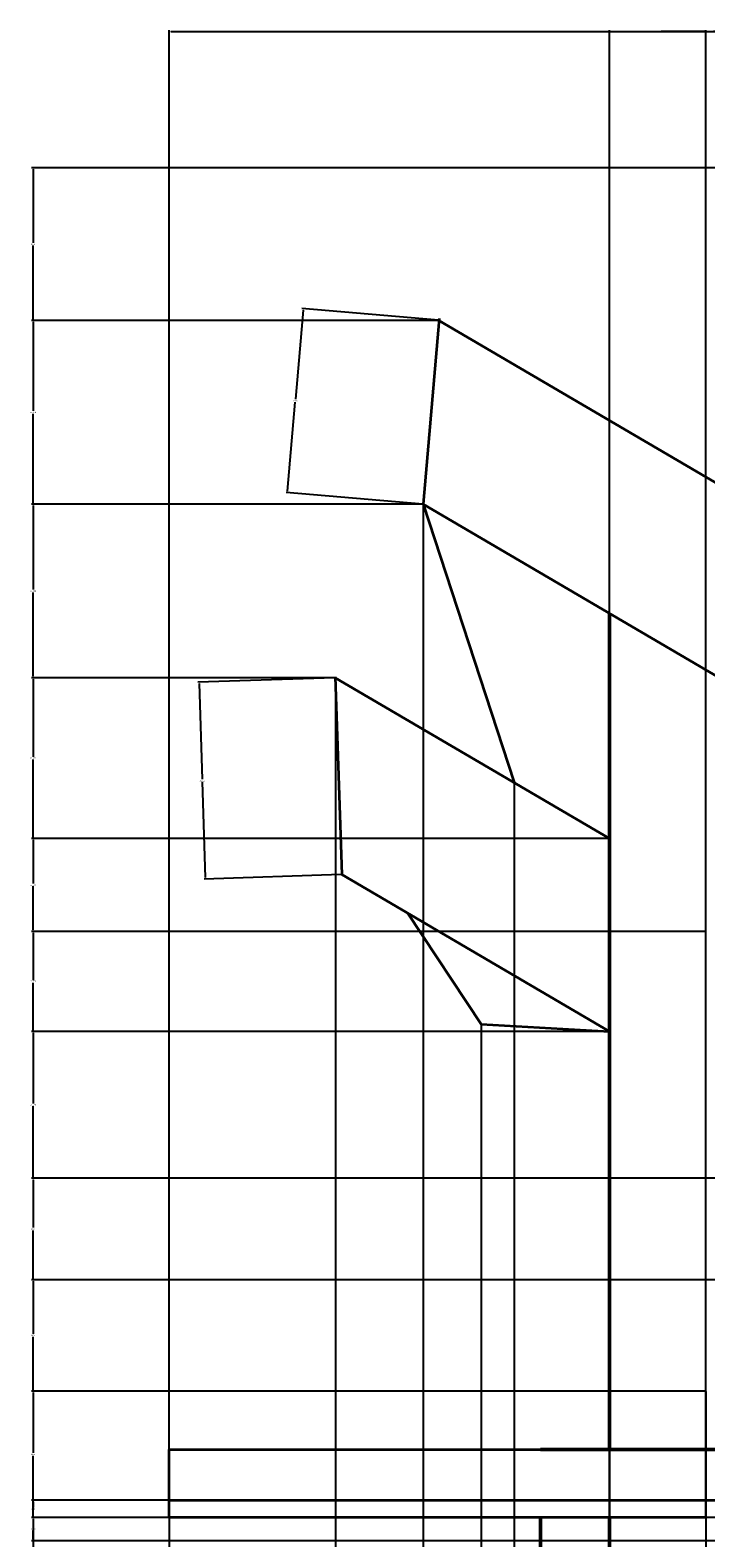
# Model space of a CAD drawing. Units: inches. Extents: x 27 to 409, y -26 to 294.
# Tile 3 of 7: x 27 to 116, y 97 to 294. Entities that reach past the tile are written whole.
import ezdxf

# ---------------------------------------------------------------- set-up
doc = ezdxf.new("R2010")
doc.units = ezdxf.units.IN
doc.header["$MEASUREMENT"] = 0
for name, color, linetype, lineweight in [('A-ANNO-DIMS', 2, 'Continuous', 18), ('A-ROOF', 1, 'Continuous', 35), ('A-WALL', 7, 'Continuous', 50)]:
    doc.layers.add(name, color=color, linetype=linetype, lineweight=lineweight)
doc.styles.get("Standard").update_dxf_attribs({"font": 'arial.ttf'})
doc.dimstyles.get("Standard").update_dxf_attribs({"dimtxt": 0.18, "dimasz": 0.18, "dimexe": 0.18, "dimexo": 0.0625, "dimgap": 0.09, "dimtad": 0, "dimtih": 1, "dimtoh": 1, "dimdec": 4, "dimzin": 0, "dimdsep": 46, "dimtxsty": 'Standard', "dimcen": 0.09, "dimadec": 0, "dimazin": 0, "dimtfac": 1, "dimtdec": 4, "dimtofl": 0, "dimtmove": 0, "dimatfit": 3, "dimfxl": 1, "dimtolj": 1, "dimtzin": 0, "dimarcsym": 0})

# ---------------------------------------------------------------- blocks, each defined once
blk = doc.blocks.new('*D7')
at = {"layer": 'A-ANNO-DIMS', "color": 0, "lineweight": -2, "transparency": 16777216}
for p, q in [((45.58, 108.44), (45.58, 293.63)), ((45.76, 293.45), (217.77, 293.45)), ((390.53, 293.45), (218.52, 293.45)), ((390.71, 136.32), (390.71, 293.63))]:
    blk.add_line(p, q, dxfattribs=at)
at = {"layer": 'A-ANNO-DIMS', "color": 0, "transparency": 16777216}
for points in [[(45.76, 293.48), (45.76, 293.42), (45.58, 293.45)], [(390.53, 293.48), (390.53, 293.42), (390.71, 293.45)]]:
    blk.add_solid(points, dxfattribs=at)
at = {"layer": 'Defpoints', "color": 0, "transparency": 16777216}
for p in [(390.71, 293.45), (390.71, 136.26), (45.58, 108.38)]:
    blk.add_point(p, dxfattribs=at)
at = {"layer": 'A-ANNO-DIMS', "color": 0, "transparency": 16777216, "insert": (218.14, 293.45), "char_height": 0.18, "attachment_point": 5}
blk.add_mtext('\\A1;345.1', dxfattribs=at)
blk = doc.blocks.new('*D8')
at = {"layer": 'A-ANNO-DIMS', "color": 0, "lineweight": -2, "transparency": 16777216}
for p, q in [((67.27, 209.05), (67.27, -26.5)), ((45.58, 99.43), (45.58, -26.5)), ((45.76, -26.32), (56.03, -26.32)), ((67.09, -26.32), (56.82, -26.32))]:
    blk.add_line(p, q, dxfattribs=at)
at = {"layer": 'A-ANNO-DIMS', "color": 0, "transparency": 16777216}
for points in [[(45.76, -26.29), (45.76, -26.35), (45.58, -26.32)], [(67.09, -26.29), (67.09, -26.35), (67.27, -26.32)]]:
    blk.add_solid(points, dxfattribs=at)
at = {"layer": 'Defpoints', "color": 0, "transparency": 16777216}
for p in [(67.27, 209.11), (45.58, 99.5), (67.27, -26.32)]:
    blk.add_point(p, dxfattribs=at)
at = {"layer": 'A-ANNO-DIMS', "color": 0, "transparency": 16777216, "insert": (56.42, -26.32), "char_height": 0.18, "attachment_point": 5}
blk.add_mtext('\\A1;21.69', dxfattribs=at)
blk = doc.blocks.new('*D9')
at = {"layer": 'A-ANNO-DIMS', "color": 0, "lineweight": -2, "transparency": 16777216}
for p, q in [((78.75, 231.7), (78.75, -26.5)), ((67.27, 209.05), (67.27, -26.5)), ((67.45, -26.32), (72.55, -26.32)), ((78.57, -26.32), (73.46, -26.32))]:
    blk.add_line(p, q, dxfattribs=at)
at = {"layer": 'A-ANNO-DIMS', "color": 0, "transparency": 16777216}
for points in [[(67.45, -26.29), (67.45, -26.35), (67.27, -26.32)], [(78.57, -26.29), (78.57, -26.35), (78.75, -26.32)]]:
    blk.add_solid(points, dxfattribs=at)
at = {"layer": 'Defpoints', "color": 0, "transparency": 16777216}
for p in [(78.75, 231.76), (67.27, 209.11), (78.75, -26.32)]:
    blk.add_point(p, dxfattribs=at)
at = {"layer": 'A-ANNO-DIMS', "color": 0, "transparency": 16777216, "insert": (73.01, -26.32), "char_height": 0.18, "attachment_point": 5}
blk.add_mtext('\\A1;11.482', dxfattribs=at)
blk = doc.blocks.new('*D10')
at = {"layer": 'A-ANNO-DIMS', "color": 0, "lineweight": -2, "transparency": 16777216}
for p, q in [((78.75, 231.7), (78.75, -26.5)), ((81.81, -8.58), (81.81, -26.5)), ((78.93, -26.32), (79.89, -26.32)), ((81.63, -26.32), (80.68, -26.32))]:
    blk.add_line(p, q, dxfattribs=at)
at = {"layer": 'A-ANNO-DIMS', "color": 0, "transparency": 16777216}
for points in [[(78.93, -26.29), (78.93, -26.35), (78.75, -26.32)], [(81.63, -26.29), (81.63, -26.35), (81.81, -26.32)]]:
    blk.add_solid(points, dxfattribs=at)
at = {"layer": 'Defpoints', "color": 0, "transparency": 16777216}
for p in [(78.75, 231.76), (81.81, -8.52), (81.81, -26.32)]:
    blk.add_point(p, dxfattribs=at)
at = {"layer": 'A-ANNO-DIMS', "color": 0, "transparency": 16777216, "insert": (80.28, -26.32), "char_height": 0.18, "attachment_point": 5}
blk.add_mtext('\\A1;3.064', dxfattribs=at)
blk = doc.blocks.new('*D11')
at = {"layer": 'A-ANNO-DIMS', "color": 0, "lineweight": -2, "transparency": 16777216}
for p, q in [((86.32, 163.84), (86.32, -26.5)), ((81.81, -8.58), (81.81, -26.5)), ((81.99, -26.32), (83.67, -26.32)), ((86.14, -26.32), (84.46, -26.32))]:
    blk.add_line(p, q, dxfattribs=at)
at = {"layer": 'A-ANNO-DIMS', "color": 0, "transparency": 16777216}
for points in [[(81.99, -26.29), (81.99, -26.35), (81.81, -26.32)], [(86.14, -26.29), (86.14, -26.35), (86.32, -26.32)]]:
    blk.add_solid(points, dxfattribs=at)
at = {"layer": 'Defpoints', "color": 0, "transparency": 16777216}
for p in [(86.32, 163.9), (81.81, -8.52), (86.32, -26.32)]:
    blk.add_point(p, dxfattribs=at)
at = {"layer": 'A-ANNO-DIMS', "color": 0, "transparency": 16777216, "insert": (84.07, -26.32), "char_height": 0.18, "attachment_point": 5}
blk.add_mtext('\\A1;4.503', dxfattribs=at)
blk = doc.blocks.new('*D12')
at = {"layer": 'A-ANNO-DIMS', "color": 0, "lineweight": -2, "transparency": 16777216}
for p, q in [((90.63, 195.36), (90.63, -26.5)), ((86.32, 163.84), (86.32, -26.5)), ((86.5, -26.32), (88.09, -26.32)), ((90.45, -26.32), (88.85, -26.32))]:
    blk.add_line(p, q, dxfattribs=at)
at = {"layer": 'A-ANNO-DIMS', "color": 0, "transparency": 16777216}
for points in [[(86.5, -26.29), (86.5, -26.35), (86.32, -26.32)], [(90.45, -26.29), (90.45, -26.35), (90.63, -26.32)]]:
    blk.add_solid(points, dxfattribs=at)
at = {"layer": 'Defpoints', "color": 0, "transparency": 16777216}
for p in [(90.63, 195.42), (86.32, 163.9), (90.63, -26.32)]:
    blk.add_point(p, dxfattribs=at)
at = {"layer": 'A-ANNO-DIMS', "color": 0, "transparency": 16777216, "insert": (88.47, -26.32), "char_height": 0.18, "attachment_point": 5}
blk.add_mtext('\\A1;4.311', dxfattribs=at)
blk = doc.blocks.new('*D13')
at = {"layer": 'A-ANNO-DIMS', "color": 0, "lineweight": -2, "transparency": 16777216}
for p, q in [((90.63, 195.36), (90.63, -26.5)), ((103.08, 162.87), (103.08, -26.5)), ((90.81, -26.32), (96.4, -26.32)), ((102.9, -26.32), (97.31, -26.32))]:
    blk.add_line(p, q, dxfattribs=at)
at = {"layer": 'A-ANNO-DIMS', "color": 0, "transparency": 16777216}
for points in [[(90.81, -26.29), (90.81, -26.35), (90.63, -26.32)], [(102.9, -26.29), (102.9, -26.35), (103.08, -26.32)]]:
    blk.add_solid(points, dxfattribs=at)
at = {"layer": 'Defpoints', "color": 0, "transparency": 16777216}
for p in [(90.63, 195.42), (103.08, 162.94), (103.08, -26.32)]:
    blk.add_point(p, dxfattribs=at)
at = {"layer": 'A-ANNO-DIMS', "color": 0, "transparency": 16777216, "insert": (96.85, -26.32), "char_height": 0.18, "attachment_point": 5}
blk.add_mtext('\\A1;12.447', dxfattribs=at)
blk = doc.blocks.new('*D14')
at = {"layer": 'A-ANNO-DIMS', "color": 0, "lineweight": -2, "transparency": 16777216}
for p, q in [((103.08, 162.87), (103.08, -26.5)), ((115.67, 115.93), (115.67, -26.5)), ((103.26, -26.32), (108.93, -26.32)), ((115.49, -26.32), (109.81, -26.32))]:
    blk.add_line(p, q, dxfattribs=at)
at = {"layer": 'A-ANNO-DIMS', "color": 0, "transparency": 16777216}
for points in [[(103.26, -26.29), (103.26, -26.35), (103.08, -26.32)], [(115.49, -26.29), (115.49, -26.35), (115.67, -26.32)]]:
    blk.add_solid(points, dxfattribs=at)
at = {"layer": 'Defpoints', "color": 0, "transparency": 16777216}
for p in [(103.08, 162.94), (115.67, 116), (115.67, -26.32)]:
    blk.add_point(p, dxfattribs=at)
at = {"layer": 'A-ANNO-DIMS', "color": 0, "transparency": 16777216, "insert": (109.37, -26.32), "char_height": 0.18, "attachment_point": 5}
blk.add_mtext('\\A1;12.591', dxfattribs=at)
blk = doc.blocks.new('*D15')
at = {"layer": 'A-ANNO-DIMS', "color": 0, "lineweight": -2, "transparency": 16777216}
for p, q in [((152.83, 275.59), (152.83, -26.5)), ((115.67, 115.93), (115.67, -26.5)), ((115.85, -26.32), (133.86, -26.32)), ((152.65, -26.32), (134.64, -26.32))]:
    blk.add_line(p, q, dxfattribs=at)
at = {"layer": 'A-ANNO-DIMS', "color": 0, "transparency": 16777216}
for points in [[(115.85, -26.29), (115.85, -26.35), (115.67, -26.32)], [(152.65, -26.29), (152.65, -26.35), (152.83, -26.32)]]:
    blk.add_solid(points, dxfattribs=at)
at = {"layer": 'Defpoints', "color": 0, "transparency": 16777216}
for p in [(152.83, 275.65), (115.67, 116), (152.83, -26.32)]:
    blk.add_point(p, dxfattribs=at)
at = {"layer": 'A-ANNO-DIMS', "color": 0, "transparency": 16777216, "insert": (134.25, -26.32), "char_height": 0.18, "attachment_point": 5}
blk.add_mtext('\\A1;37.17', dxfattribs=at)
blk = doc.blocks.new('*D28')
at = {"layer": 'A-ANNO-DIMS', "color": 0, "lineweight": -2, "transparency": 16777216}
for p, q in [((45.51, 99.5), (27.6, 99.5)), ((27.78, 99.32), (27.78, 69.78)), ((27.78, 39.89), (27.78, 69.42)), ((115.6, 39.71), (27.6, 39.71))]:
    blk.add_line(p, q, dxfattribs=at)
at = {"layer": 'A-ANNO-DIMS', "color": 0, "transparency": 16777216}
for points in [[(27.75, 99.32), (27.81, 99.32), (27.78, 99.5)], [(27.75, 39.89), (27.81, 39.89), (27.78, 39.71)]]:
    blk.add_solid(points, dxfattribs=at)
at = {"layer": 'Defpoints', "color": 0, "transparency": 16777216}
for p in [(27.78, 99.5), (45.58, 99.5), (115.67, 39.71)]:
    blk.add_point(p, dxfattribs=at)
at = {"layer": 'A-ANNO-DIMS', "color": 0, "transparency": 16777216, "insert": (27.78, 69.6), "char_height": 0.18, "attachment_point": 5}
blk.add_mtext('\\A1;59.79', dxfattribs=at)
blk = doc.blocks.new('*D29')
at = {"layer": 'A-ANNO-DIMS', "color": 0, "lineweight": -2, "transparency": 16777216}
for p, q in [((115.6, 116), (27.6, 116)), ((27.78, 115.82), (27.78, 107.93)), ((27.78, 99.68), (27.78, 107.56)), ((45.51, 99.5), (27.6, 99.5))]:
    blk.add_line(p, q, dxfattribs=at)
at = {"layer": 'A-ANNO-DIMS', "color": 0, "transparency": 16777216}
for points in [[(27.75, 115.82), (27.81, 115.82), (27.78, 116)], [(27.75, 99.68), (27.81, 99.68), (27.78, 99.5)]]:
    blk.add_solid(points, dxfattribs=at)
at = {"layer": 'Defpoints', "color": 0, "transparency": 16777216}
for p in [(27.78, 116), (115.67, 116), (45.58, 99.5)]:
    blk.add_point(p, dxfattribs=at)
at = {"layer": 'A-ANNO-DIMS', "color": 0, "transparency": 16777216, "insert": (27.78, 107.75), "char_height": 0.18, "attachment_point": 5}
blk.add_mtext('\\A1;16.5', dxfattribs=at)
blk = doc.blocks.new('*D30')
at = {"layer": 'A-ANNO-DIMS', "color": 0, "lineweight": -2, "transparency": 16777216}
for p, q in [((206.63, 130.53), (27.6, 130.53)), ((27.78, 130.35), (27.78, 123.45)), ((27.78, 116.18), (27.78, 123.08)), ((115.6, 116), (27.6, 116))]:
    blk.add_line(p, q, dxfattribs=at)
at = {"layer": 'A-ANNO-DIMS', "color": 0, "transparency": 16777216}
for points in [[(27.75, 130.35), (27.81, 130.35), (27.78, 130.53)], [(27.75, 116.18), (27.81, 116.18), (27.78, 116)]]:
    blk.add_solid(points, dxfattribs=at)
at = {"layer": 'Defpoints', "color": 0, "transparency": 16777216}
for p in [(27.78, 130.53), (206.7, 130.53), (115.67, 116)]:
    blk.add_point(p, dxfattribs=at)
at = {"layer": 'A-ANNO-DIMS', "color": 0, "transparency": 16777216, "insert": (27.78, 123.26), "char_height": 0.18, "attachment_point": 5}
blk.add_mtext('\\A1;14.54', dxfattribs=at)
blk = doc.blocks.new('*D31')
at = {"layer": 'A-ANNO-DIMS', "color": 0, "lineweight": -2, "transparency": 16777216}
for p, q in [((210.03, 143.77), (27.6, 143.77)), ((27.78, 143.59), (27.78, 137.34)), ((27.78, 130.71), (27.78, 136.97)), ((206.63, 130.53), (27.6, 130.53))]:
    blk.add_line(p, q, dxfattribs=at)
at = {"layer": 'A-ANNO-DIMS', "color": 0, "transparency": 16777216}
for points in [[(27.75, 143.59), (27.81, 143.59), (27.78, 143.77)], [(27.75, 130.71), (27.81, 130.71), (27.78, 130.53)]]:
    blk.add_solid(points, dxfattribs=at)
at = {"layer": 'Defpoints', "color": 0, "transparency": 16777216}
for p in [(27.78, 143.77), (210.09, 143.77), (206.7, 130.53)]:
    blk.add_point(p, dxfattribs=at)
at = {"layer": 'A-ANNO-DIMS', "color": 0, "transparency": 16777216, "insert": (27.78, 137.15), "char_height": 0.18, "attachment_point": 5}
blk.add_mtext('\\A1;13.24', dxfattribs=at)
blk = doc.blocks.new('*D32')
at = {"layer": 'A-ANNO-DIMS', "color": 0, "lineweight": -2, "transparency": 16777216}
for p, q in [((103.01, 162.94), (27.6, 162.94)), ((27.78, 162.76), (27.78, 153.54)), ((27.78, 143.95), (27.78, 153.17)), ((210.03, 143.77), (27.6, 143.77))]:
    blk.add_line(p, q, dxfattribs=at)
at = {"layer": 'A-ANNO-DIMS', "color": 0, "transparency": 16777216}
for points in [[(27.75, 162.76), (27.81, 162.76), (27.78, 162.94)], [(27.75, 143.95), (27.81, 143.95), (27.78, 143.77)]]:
    blk.add_solid(points, dxfattribs=at)
at = {"layer": 'Defpoints', "color": 0, "transparency": 16777216}
for p in [(27.78, 162.94), (103.08, 162.94), (210.09, 143.77)]:
    blk.add_point(p, dxfattribs=at)
at = {"layer": 'A-ANNO-DIMS', "color": 0, "transparency": 16777216, "insert": (27.78, 153.36), "char_height": 0.18, "attachment_point": 5}
blk.add_mtext('\\A1;19.164', dxfattribs=at)
blk = doc.blocks.new('*D33')
at = {"layer": 'A-ANNO-DIMS', "color": 0, "lineweight": -2, "transparency": 16777216}
for p, q in [((115.6, 176), (27.6, 176)), ((27.78, 175.82), (27.78, 169.65)), ((27.78, 163.12), (27.78, 169.28)), ((103.01, 162.94), (27.6, 162.94))]:
    blk.add_line(p, q, dxfattribs=at)
at = {"layer": 'A-ANNO-DIMS', "color": 0, "transparency": 16777216}
for points in [[(27.75, 175.82), (27.81, 175.82), (27.78, 176)], [(27.75, 163.12), (27.81, 163.12), (27.78, 162.94)]]:
    blk.add_solid(points, dxfattribs=at)
at = {"layer": 'Defpoints', "color": 0, "transparency": 16777216}
for p in [(27.78, 176), (115.67, 176), (103.08, 162.94)]:
    blk.add_point(p, dxfattribs=at)
at = {"layer": 'A-ANNO-DIMS', "color": 0, "transparency": 16777216, "insert": (27.78, 169.47), "char_height": 0.18, "attachment_point": 5}
blk.add_mtext('\\A1;13.058', dxfattribs=at)
blk = doc.blocks.new('*D34')
at = {"layer": 'A-ANNO-DIMS', "color": 0, "lineweight": -2, "transparency": 16777216}
for p, q in [((103.01, 188.13), (27.6, 188.13)), ((27.78, 187.95), (27.78, 182.24)), ((27.78, 176.18), (27.78, 181.88)), ((115.6, 176), (27.6, 176))]:
    blk.add_line(p, q, dxfattribs=at)
at = {"layer": 'A-ANNO-DIMS', "color": 0, "transparency": 16777216}
for points in [[(27.75, 187.95), (27.81, 187.95), (27.78, 188.13)], [(27.75, 176.18), (27.81, 176.18), (27.78, 176)]]:
    blk.add_solid(points, dxfattribs=at)
at = {"layer": 'Defpoints', "color": 0, "transparency": 16777216}
for p in [(27.78, 188.13), (103.08, 188.13), (115.67, 176)]:
    blk.add_point(p, dxfattribs=at)
at = {"layer": 'A-ANNO-DIMS', "color": 0, "transparency": 16777216, "insert": (27.78, 182.06), "char_height": 0.18, "attachment_point": 5}
blk.add_mtext('\\A1;12.136', dxfattribs=at)
blk = doc.blocks.new('*D35')
at = {"layer": 'A-ANNO-DIMS', "color": 0, "lineweight": -2, "transparency": 16777216}
for p, q in [((67.21, 209.11), (27.6, 209.11)), ((27.78, 208.93), (27.78, 198.8)), ((27.78, 188.31), (27.78, 198.44)), ((103.01, 188.13), (27.6, 188.13))]:
    blk.add_line(p, q, dxfattribs=at)
at = {"layer": 'A-ANNO-DIMS', "color": 0, "transparency": 16777216}
for points in [[(27.75, 208.93), (27.81, 208.93), (27.78, 209.11)], [(27.75, 188.31), (27.81, 188.31), (27.78, 188.13)]]:
    blk.add_solid(points, dxfattribs=at)
at = {"layer": 'Defpoints', "color": 0, "transparency": 16777216}
for p in [(27.78, 209.11), (67.27, 209.11), (103.08, 188.13)]:
    blk.add_point(p, dxfattribs=at)
at = {"layer": 'A-ANNO-DIMS', "color": 0, "transparency": 16777216, "insert": (27.78, 198.62), "char_height": 0.18, "attachment_point": 5}
blk.add_mtext('\\A1;20.983', dxfattribs=at)
blk = doc.blocks.new('*D36')
at = {"layer": 'A-ANNO-DIMS', "color": 0, "lineweight": -2, "transparency": 16777216}
for p, q in [((78.69, 231.76), (27.6, 231.76)), ((27.78, 231.58), (27.78, 220.62)), ((27.78, 209.29), (27.78, 220.25)), ((67.21, 209.11), (27.6, 209.11))]:
    blk.add_line(p, q, dxfattribs=at)
at = {"layer": 'A-ANNO-DIMS', "color": 0, "transparency": 16777216}
for points in [[(27.75, 231.58), (27.81, 231.58), (27.78, 231.76)], [(27.75, 209.29), (27.81, 209.29), (27.78, 209.11)]]:
    blk.add_solid(points, dxfattribs=at)
at = {"layer": 'Defpoints', "color": 0, "transparency": 16777216}
for p in [(27.78, 231.76), (78.75, 231.76), (67.27, 209.11)]:
    blk.add_point(p, dxfattribs=at)
at = {"layer": 'A-ANNO-DIMS', "color": 0, "transparency": 16777216, "insert": (27.78, 220.44), "char_height": 0.18, "attachment_point": 5}
blk.add_mtext('\\A1;22.644', dxfattribs=at)
blk = doc.blocks.new('*D37')
at = {"layer": 'A-ANNO-DIMS', "color": 0, "lineweight": -2, "transparency": 16777216}
for p, q in [((80.73, 255.75), (27.6, 255.75)), ((27.78, 255.57), (27.78, 243.94)), ((27.78, 231.94), (27.78, 243.57)), ((78.69, 231.76), (27.6, 231.76))]:
    blk.add_line(p, q, dxfattribs=at)
at = {"layer": 'A-ANNO-DIMS', "color": 0, "transparency": 16777216}
for points in [[(27.75, 255.57), (27.81, 255.57), (27.78, 255.75)], [(27.75, 231.94), (27.81, 231.94), (27.78, 231.76)]]:
    blk.add_solid(points, dxfattribs=at)
at = {"layer": 'Defpoints', "color": 0, "transparency": 16777216}
for p in [(27.78, 255.75), (80.8, 255.75), (78.75, 231.76)]:
    blk.add_point(p, dxfattribs=at)
at = {"layer": 'A-ANNO-DIMS', "color": 0, "transparency": 16777216, "insert": (27.78, 243.76), "char_height": 0.18, "attachment_point": 5}
blk.add_mtext('\\A1;23.994', dxfattribs=at)
blk = doc.blocks.new('*D38')
at = {"layer": 'A-ANNO-DIMS', "color": 0, "lineweight": -2, "transparency": 16777216}
for p, q in [((152.77, 275.65), (27.6, 275.65)), ((27.78, 275.47), (27.78, 265.88)), ((27.78, 255.93), (27.78, 265.52)), ((80.73, 255.75), (27.6, 255.75))]:
    blk.add_line(p, q, dxfattribs=at)
at = {"layer": 'A-ANNO-DIMS', "color": 0, "transparency": 16777216}
for points in [[(27.75, 275.47), (27.81, 275.47), (27.78, 275.65)], [(27.75, 255.93), (27.81, 255.93), (27.78, 255.75)]]:
    blk.add_solid(points, dxfattribs=at)
at = {"layer": 'Defpoints', "color": 0, "transparency": 16777216}
for p in [(27.78, 275.65), (152.83, 275.65), (80.8, 255.75)]:
    blk.add_point(p, dxfattribs=at)
at = {"layer": 'A-ANNO-DIMS', "color": 0, "transparency": 16777216, "insert": (27.78, 265.7), "char_height": 0.18, "attachment_point": 5}
blk.add_mtext('\\A1;19.9', dxfattribs=at)
blk = doc.blocks.new('*D49')
at = {"layer": 'A-ANNO-DIMS', "color": 0, "lineweight": -2, "transparency": 16777216}
for p, q in [((63.05, 257.09), (62.05, 245.45)), ((80.73, 255.76), (62.88, 257.28)), ((61.03, 233.45), (62.02, 245.09)), ((78.69, 231.76), (60.83, 233.29))]:
    blk.add_line(p, q, dxfattribs=at)
at = {"layer": 'A-ANNO-DIMS', "color": 0, "transparency": 16777216}
for points in [[(63.02, 257.09), (63.08, 257.08), (63.06, 257.27)], [(61, 233.45), (61.06, 233.45), (61.01, 233.27)]]:
    blk.add_solid(points, dxfattribs=at)
at = {"layer": 'Defpoints', "color": 0, "transparency": 16777216}
for p in [(63.06, 257.27), (80.8, 255.75), (78.75, 231.76)]:
    blk.add_point(p, dxfattribs=at)
at = {"layer": 'A-ANNO-DIMS', "color": 0, "transparency": 16777216, "insert": (62.04, 245.27), "char_height": 0.18, "attachment_point": 5}
blk.add_mtext('\\A1;24.08', dxfattribs=at)
blk = doc.blocks.new('*D50')
at = {"layer": 'A-ANNO-DIMS', "color": 0, "lineweight": -2, "transparency": 16777216}
for p, q in [((67.21, 209.11), (49.3, 208.52)), ((49.48, 208.35), (49.89, 195.87)), ((50.32, 183.02), (49.91, 195.5)), ((68.05, 183.42), (50.14, 182.83))]:
    blk.add_line(p, q, dxfattribs=at)
at = {"layer": 'A-ANNO-DIMS', "color": 0, "transparency": 16777216}
for points in [[(49.51, 208.35), (49.45, 208.35), (49.48, 208.53)], [(50.35, 183.02), (50.29, 183.02), (50.32, 182.84)]]:
    blk.add_solid(points, dxfattribs=at)
at = {"layer": 'Defpoints', "color": 0, "transparency": 16777216}
for p in [(67.27, 209.11), (49.48, 208.53), (68.11, 183.43)]:
    blk.add_point(p, dxfattribs=at)
at = {"layer": 'A-ANNO-DIMS', "color": 0, "transparency": 16777216, "insert": (49.9, 195.68), "char_height": 0.18, "attachment_point": 5}
blk.add_mtext('\\A1;25.703', dxfattribs=at)
blk = doc.blocks.new('*D72')
at = {"layer": 'A-ANNO-DIMS', "color": 0, "lineweight": -2, "transparency": 16777216}
for p, q in [((190.01, 99.5), (27.6, 99.5)), ((27.78, 99.32), (27.78, 98.17)), ((196.04, 96.47), (27.6, 96.47)), ((27.78, 96.65), (27.78, 97.8))]:
    blk.add_line(p, q, dxfattribs=at)
at = {"layer": 'A-ANNO-DIMS', "color": 0, "transparency": 16777216}
for points in [[(27.75, 99.32), (27.81, 99.32), (27.78, 99.5)], [(27.75, 96.65), (27.81, 96.65), (27.78, 96.47)]]:
    blk.add_solid(points, dxfattribs=at)
at = {"layer": 'Defpoints', "color": 0, "transparency": 16777216}
for p in [(27.78, 99.5), (190.08, 99.5), (196.1, 96.47)]:
    blk.add_point(p, dxfattribs=at)
at = {"layer": 'A-ANNO-DIMS', "color": 0, "transparency": 16777216, "insert": (27.78, 97.98), "char_height": 0.18, "attachment_point": 5}
blk.add_mtext('\\A1;3.023', dxfattribs=at)
blk = doc.blocks.new('*D73')
at = {"layer": 'A-ANNO-DIMS', "color": 0, "lineweight": -2, "transparency": 16777216}
for p, q in [((229.04, 101.74), (27.6, 101.74)), ((27.78, 101.56), (27.78, 100.8)), ((27.78, 99.68), (27.78, 100.44)), ((190.01, 99.5), (27.6, 99.5))]:
    blk.add_line(p, q, dxfattribs=at)
at = {"layer": 'A-ANNO-DIMS', "color": 0, "transparency": 16777216}
for points in [[(27.75, 101.56), (27.81, 101.56), (27.78, 101.74)], [(27.75, 99.68), (27.81, 99.68), (27.78, 99.5)]]:
    blk.add_solid(points, dxfattribs=at)
at = {"layer": 'Defpoints', "color": 0, "transparency": 16777216}
for p in [(27.78, 101.74), (229.1, 101.74), (190.08, 99.5)]:
    blk.add_point(p, dxfattribs=at)
at = {"layer": 'A-ANNO-DIMS', "color": 0, "transparency": 16777216, "insert": (27.78, 100.62), "char_height": 0.18, "attachment_point": 5}
blk.add_mtext('\\A1;2.24', dxfattribs=at)
blk = doc.blocks.new('*D96')
at = {"layer": 'A-ANNO-DIMS', "color": 0, "lineweight": -2, "transparency": 16777216}
for p, q in [((103.08, 39.77), (103.08, 293.63)), ((103.26, 293.45), (108.93, 293.45)), ((115.49, 293.45), (109.81, 293.45)), ((115.67, 99.56), (115.67, 293.63))]:
    blk.add_line(p, q, dxfattribs=at)
at = {"layer": 'A-ANNO-DIMS', "color": 0, "transparency": 16777216}
for points in [[(103.26, 293.48), (103.26, 293.42), (103.08, 293.45)], [(115.49, 293.48), (115.49, 293.42), (115.67, 293.45)]]:
    blk.add_solid(points, dxfattribs=at)
at = {"layer": 'Defpoints', "color": 0, "transparency": 16777216}
for p in [(115.67, 293.45), (115.67, 99.5), (103.08, 39.71)]:
    blk.add_point(p, dxfattribs=at)
at = {"layer": 'A-ANNO-DIMS', "color": 0, "transparency": 16777216, "insert": (109.37, 293.45), "char_height": 0.18, "attachment_point": 5}
blk.add_mtext('\\A1;12.591', dxfattribs=at)
blk = doc.blocks.new('*D97')
at = {"layer": 'A-ANNO-DIMS', "color": 0, "lineweight": -2, "transparency": 16777216}
for p, q in [((115.67, 99.56), (115.67, 293.63)), ((115.85, 293.45), (116.17, 293.45)), ((116.99, 293.45), (116.66, 293.45)), ((117.17, 98.27), (117.17, 293.63))]:
    blk.add_line(p, q, dxfattribs=at)
at = {"layer": 'A-ANNO-DIMS', "color": 0, "transparency": 16777216}
for points in [[(115.85, 293.48), (115.85, 293.42), (115.67, 293.45)], [(116.99, 293.48), (116.99, 293.42), (117.17, 293.45)]]:
    blk.add_solid(points, dxfattribs=at)
at = {"layer": 'Defpoints', "color": 0, "transparency": 16777216}
for p in [(117.17, 293.45), (115.67, 99.5), (117.17, 98.21)]:
    blk.add_point(p, dxfattribs=at)
at = {"layer": 'A-ANNO-DIMS', "color": 0, "transparency": 16777216, "insert": (116.42, 293.45), "char_height": 0.18, "attachment_point": 5}
blk.add_mtext('\\A1;1.5', dxfattribs=at)

msp = doc.modelspace()

# ---------------------------------------------------------------- linework, layer by layer
at = {"layer": 'A-ROOF'}
for p, q in [((80.8174, 255.9907), (78.7499, 231.7582)), ((78.7499, 231.7582), (90.6277, 195.4248)), ((67.264, 209.2221), (68.1126, 183.4252)), ((76.6837, 178.4025), (86.3168, 163.9028)), ((86.3168, 163.9028), (86.3168, 163.9028)), ((86.3168, 163.9028), (103.0751, 162.937)), ((45.5772, 101.7396), (229.1036, 101.7396))]:
    msp.add_line(p, q, dxfattribs=at)
for points in [[(166.0751, 205.7788), (80.7971, 255.7521)], [(78.7499, 231.7582), (166.0751, 180.5852)], [(103.0751, 188.1307), (67.2675, 209.1141)], [(68.1126, 183.4252), (103.0751, 162.937)], [(115.6666, 99.4952), (45.5772, 99.4952), (45.5772, 108.3803), (229.1036, 108.3803), (229.1036, 99.4952), (166.0751, 99.4952)]]:
    msp.add_lwpolyline(points, dxfattribs=at)
at = {"layer": 'A-WALL'}
for p, q in [((103.0751, 217.5035), (103.0751, 108.3803)), ((94.0751, 99.4952), (94.0751, 15.4825)), ((103.0751, 99.4952), (103.0751, 15.4825))]:
    msp.add_line(p, q, dxfattribs=at)
msp.add_lwpolyline([(334.0751, 144.2493), (334.0751, 108.3803), (94.0751, 108.3803)], dxfattribs=at)

# ---------------------------------------------------------------- dimensions: what is measured, and where the dimension line sits
at = {"layer": 'A-ANNO-DIMS'}
for base, p1, p2, override, picture, middle in [((390.7054, 293.4517), (45.5772, 108.3803), (390.7054, 136.2572), {"dimdec": 1, "dimlfac": 1, "dimrnd": 0, "dimzin": 0, "dimdsep": 46, "dimlunit": 2}, '*D7', (218.1413, 293.4517)), ((115.66655, 293.45166), (103.07506, 39.70931), (115.66655, 99.49521), {"dimdec": 3, "dimlfac": 1, "dimrnd": 0, "dimzin": 0, "dimdsep": 46, "dimlunit": 2}, '*D96', (109.3708, 293.45166)), ((117.1666, 293.4517), (115.6666, 99.4952), (117.1666, 98.2093), {"dimdec": 1, "dimlfac": 1, "dimrnd": 0, "dimzin": 0, "dimdsep": 46, "dimlunit": 2}, '*D97', (116.4166, 293.4517)), ((152.833, -26.3175), (115.6666, 115.9951), (152.833, 275.6517), {"dimdec": 2, "dimlfac": 1, "dimrnd": 0, "dimzin": 0, "dimdsep": 46, "dimlunit": 2}, '*D15', (134.2498, -26.3175)), ((78.7499, -26.3175), (67.2675, 209.1141), (78.7499, 231.7582), {"dimdec": 3, "dimlfac": 1, "dimrnd": 0, "dimzin": 0, "dimdsep": 46, "dimlunit": 2}, '*D9', (73.0087, -26.3175)), ((81.814, -26.3175), (78.7499, 231.7582), (81.814, -8.5175), {"dimdec": 3, "dimlfac": 1, "dimrnd": 0, "dimzin": 0, "dimdsep": 46, "dimlunit": 2}, '*D10', (80.2819, -26.3175)), ((67.2675, -26.3175), (45.5772, 99.4952), (67.2675, 209.1141), {"dimdec": 2, "dimlfac": 1, "dimrnd": 0, "dimzin": 0, "dimdsep": 46, "dimlunit": 2}, '*D8', (56.4224, -26.3175)), ((90.6277, -26.3175), (86.3168, 163.9028), (90.6277, 195.4248), {"dimdec": 3, "dimlfac": 1, "dimrnd": 0, "dimzin": 0, "dimdsep": 46, "dimlunit": 2}, '*D12', (88.4723, -26.3175)), ((103.0751, -26.3175), (90.6277, 195.4248), (103.0751, 162.937), {"dimdec": 3, "dimlfac": 1, "dimrnd": 0, "dimzin": 0, "dimdsep": 46, "dimlunit": 2}, '*D13', (96.8514, -26.3175)), ((86.3168, -26.3175), (81.814, -8.5175), (86.3168, 163.9028), {"dimdec": 3, "dimlfac": 1, "dimrnd": 0, "dimzin": 0, "dimdsep": 46, "dimlunit": 2}, '*D11', (84.0654, -26.3175)), ((115.66655, -26.31755), (103.07506, 162.93703), (115.66655, 115.99512), {"dimdec": 3, "dimlfac": 1, "dimrnd": 0, "dimzin": 0, "dimdsep": 46, "dimlunit": 2}, '*D14', (109.3708, -26.31755))]:
    dim = msp.add_linear_dim(base=base, p1=p1, p2=p2, dimstyle='Standard', override=override, dxfattribs=at)
    dim.commit()
    dim.dimension.update_dxf_attribs({"geometry": picture, "text_midpoint": middle})
for base, p1, p2, angle, override, picture, middle in [((27.7772, 275.6517), (80.7971, 255.7521), (152.833, 275.6517), 90, {"dimdec": 1, "dimlfac": 1, "dimrnd": 0, "dimzin": 0, "dimdsep": 46, "dimlunit": 2}, '*D38', (27.7772, 265.7019)), ((63.0615, 257.2653), (78.7499, 231.7582), (80.7971, 255.7521), 85.123198, {"dimdec": 2, "dimlfac": 1, "dimrnd": 0, "dimzin": 0, "dimdsep": 46, "dimlunit": 2}, '*D49', (62.0379, 245.2684)), ((27.7772, 255.7521), (78.7499, 231.7582), (80.7971, 255.7521), 90, {"dimdec": 3, "dimlfac": 1, "dimrnd": 0, "dimzin": 0, "dimdsep": 46, "dimlunit": 2}, '*D37', (27.7772, 243.7551)), ((27.7772, 231.7582), (67.2675, 209.1141), (78.7499, 231.7582), 90, {"dimdec": 3, "dimlfac": 1, "dimrnd": 0, "dimzin": 0, "dimdsep": 46, "dimlunit": 2}, '*D36', (27.7772, 220.4361)), ((27.7772, 209.1141), (103.0751, 188.1307), (67.2675, 209.1141), 90, {"dimdec": 3, "dimlfac": 1, "dimrnd": 0, "dimzin": 0, "dimdsep": 46, "dimlunit": 2}, '*D35', (27.7772, 198.6224)), ((49.4771, 208.5288), (68.1126, 183.4252), (67.2675, 209.1141), 91.884134, {"dimdec": 3, "dimlfac": 1, "dimrnd": 0, "dimzin": 0, "dimdsep": 46, "dimlunit": 2}, '*D50', (49.8997, 195.6844)), ((27.7772, 188.1307), (115.6666, 175.9951), (103.0751, 188.1307), 90, {"dimdec": 3, "dimlfac": 1, "dimrnd": 0, "dimzin": 0, "dimdsep": 46, "dimlunit": 2}, '*D34', (27.7772, 182.0629)), ((27.7772, 175.9951), (103.0751, 162.937), (115.6666, 175.9951), 90, {"dimdec": 3, "dimlfac": 1, "dimrnd": 0, "dimzin": 0, "dimdsep": 46, "dimlunit": 2}, '*D33', (27.7772, 169.4661)), ((27.7772, 162.937), (210.0897, 143.7732), (103.0751, 162.937), 90, {"dimdec": 3, "dimlfac": 1, "dimrnd": 0, "dimzin": 0, "dimdsep": 46, "dimlunit": 2}, '*D32', (27.7772, 153.3551)), ((27.7772, 143.7732), (206.6961, 130.5342), (210.0897, 143.7732), 90, {"dimdec": 2, "dimlfac": 1, "dimrnd": 0, "dimzin": 0, "dimdsep": 46, "dimlunit": 2}, '*D31', (27.7772, 137.1537)), ((27.7772, 130.5342), (115.6666, 115.9951), (206.6961, 130.5342), 90, {"dimdec": 2, "dimlfac": 1, "dimrnd": 0, "dimzin": 0, "dimdsep": 46, "dimlunit": 2}, '*D30', (27.7772, 123.2647)), ((27.7772, 115.9951), (45.5772, 99.4952), (115.6666, 115.9951), 90, {"dimdec": 1, "dimlfac": 1, "dimrnd": 0, "dimzin": 0, "dimdsep": 46, "dimlunit": 2}, '*D29', (27.7772, 107.7452)), ((27.7772, 101.7396), (190.0751, 99.4952), (229.1036, 101.7396), 90, {"dimdec": 2, "dimlfac": 1, "dimrnd": 0, "dimzin": 0, "dimdsep": 46, "dimlunit": 2}, '*D73', (27.7772, 100.6174)), ((27.7772, 99.4952), (115.6666, 39.7093), (45.5772, 99.4952), 90, {"dimdec": 2, "dimlfac": 1, "dimrnd": 0, "dimzin": 0, "dimdsep": 46, "dimlunit": 2}, '*D28', (27.7772, 69.6023)), ((27.7772, 99.4952), (196.1036, 96.4722), (190.0751, 99.4952), 90, {"dimdec": 3, "dimlfac": 1, "dimrnd": 0, "dimzin": 0, "dimdsep": 46, "dimlunit": 2}, '*D72', (27.7772, 97.9837))]:
    dim = msp.add_linear_dim(base=base, p1=p1, p2=p2, angle=angle, dimstyle='Standard', override=override, dxfattribs=at)
    dim.commit()
    dim.dimension.update_dxf_attribs({"geometry": picture, "text_midpoint": middle})

doc.saveas('drawing.dxf')
